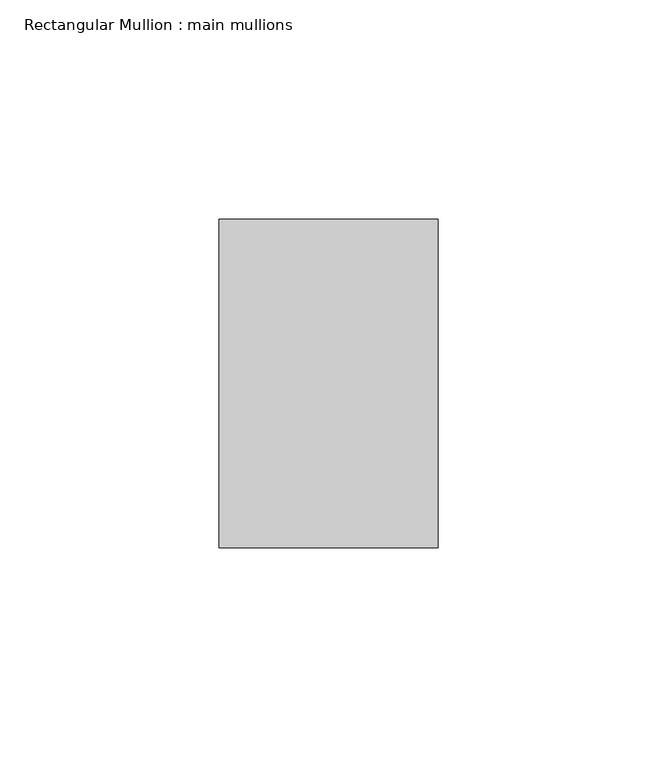
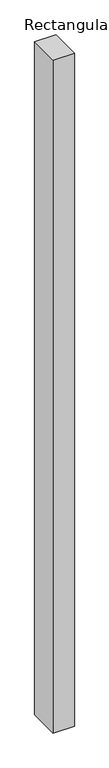
"""IFC4 building model written with IfcOpenShell, lengths in millimetres: member geometry, Rectangular Mullion : main mullions."""

from ifc_helpers import new_model, si_unit, frame, origin, place, context, project, spatial, polyline, outline, extrude, source, transform, mapped, element, save


def rectangular_mullion_main_mullions_4e228a20(model_context):
    return source(origin(), model_context, "Body", "SweptSolid", [
        extrude(outline(polyline([(25.0, 37.5), (25.0, -37.5), (-25.0, -37.5), (-25.0, 37.5), (25.0, 37.5)])), frame((0.0, 0.0, -1675.0), z_axis=(0.0, 0.0, 1.0), x_axis=(1.0, 0.0, 0.0)), (0.0, 0.0, 1.0), 1675.0),
    ])


if __name__ == "__main__":
    model = new_model("IFC4")
    model_context = context("Model", 3, world=origin())
    ifc_project = project(units=[si_unit("LENGTHUNIT", "METRE", prefix="MILLI")], contexts=[model_context])
    site = spatial("IfcSite", under=ifc_project)
    building = spatial("IfcBuilding", under=site)
    placement = place(None, origin())
    rectangular_mullion_main_mullions_shape = rectangular_mullion_main_mullions_4e228a20(model_context)
    element("IfcMember", 1, ObjectType="Rectangular Mullion : main mullions", at=placement, inside=building, context=model_context, shape_type="MappedRepresentation", body=[
        mapped(rectangular_mullion_main_mullions_shape, transform((0.0, 0.0, 0.0), x_axis=(1.0, 0.0, 0.0), y_axis=(0.0, 1.0, 0.0), z_axis=(0.0, 0.0, 1.0))),
    ])
    save(model, "model.ifc")

# Revit data of these elements
# Type "Rectangular Mullion : main mullions"
#   built-in parameter 1007304 = 0.246063 (stored number, unit not read)
#   built-in parameter 1007301 = 0.082021 (stored number, unit not read)
#   built-in parameter 1007300 = 0.082021 (stored number, unit not read)
# Element 1 (IfcMember, "Rectangular Mullion : main mullions")
#   Materials on its faces: "Aluminum"
# Materials
#   "Aluminum": class "Metal", colour RGB 136 136 136, transparency 0, Description = "Aluminum 6061", Cost = 0
